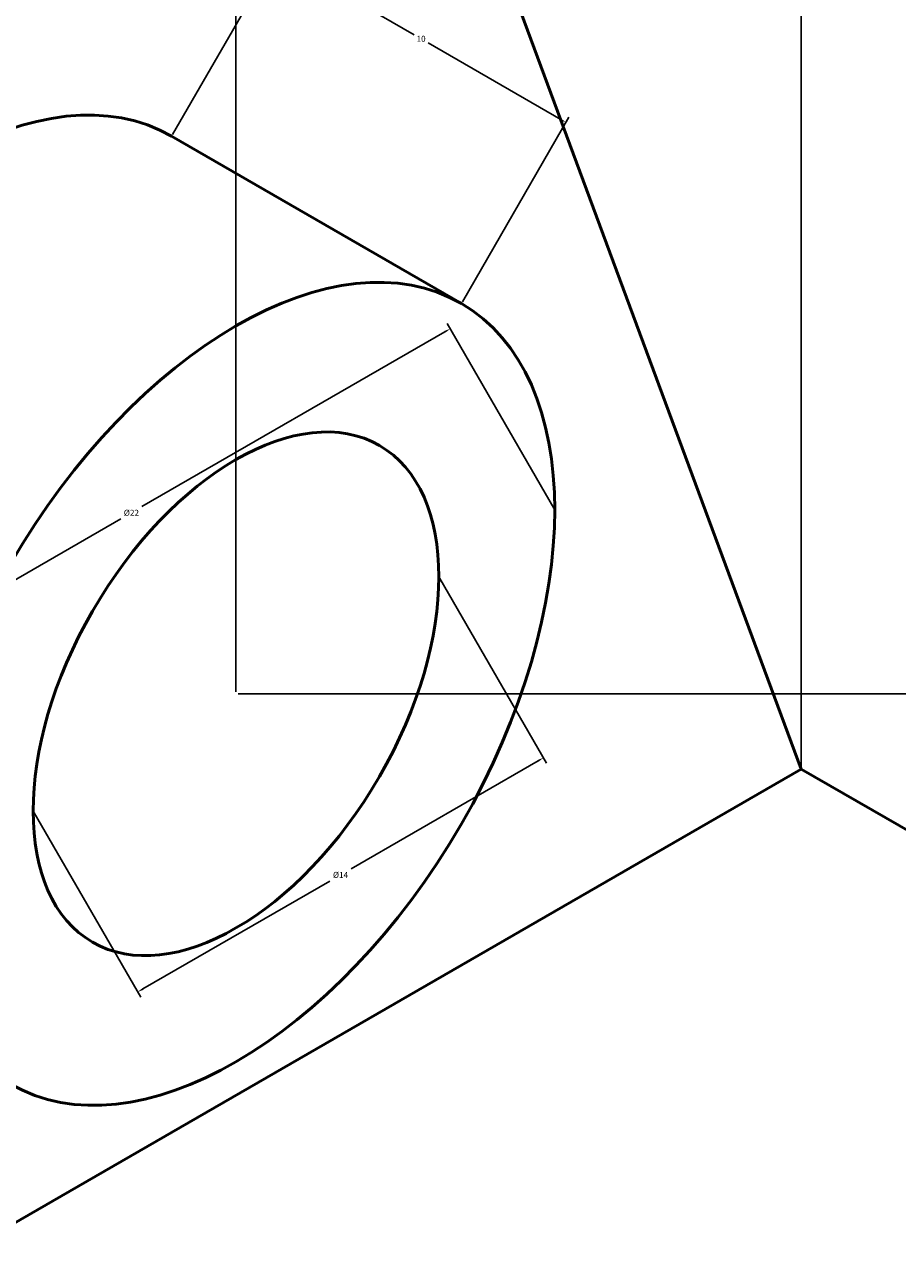
# Model space of a CAD drawing. Units: inches. Extents: x -23 to 69, y -27 to 96.
# Tile 7 of 10: x 11 to 37, y 35 to 72. Entities that reach past the tile are written whole.
import ezdxf

# ---------------------------------------------------------------- set-up
doc = ezdxf.new("R2010")
doc.units = ezdxf.units.IN
doc.header["$MEASUREMENT"] = 0
doc.layers.add('M-DIMS', color=2, linetype='Continuous', lineweight=18)
doc.layers.add('M-OUTL', color=7, linetype='Continuous', lineweight=50)
doc.styles.get("Standard").update_dxf_attribs({"font": 'arial.ttf'})
doc.dimstyles.get("Standard").update_dxf_attribs({"dimtxt": 0.18, "dimasz": 0.18, "dimexe": 0.18, "dimexo": 0.0625, "dimgap": 0.09, "dimtad": 0, "dimtih": 1, "dimtoh": 1, "dimdec": 4, "dimzin": 0, "dimdsep": 46, "dimtxsty": 'Standard', "dimcen": 0.09, "dimadec": 0, "dimazin": 0, "dimtfac": 1, "dimtdec": 4, "dimtofl": 0, "dimtmove": 0, "dimatfit": 3, "dimfxl": 1, "dimtolj": 1, "dimtzin": 0, "dimarcsym": 0})

# ---------------------------------------------------------------- blocks, each defined once
blk = doc.blocks.new('*D1')
at = {"layer": 'Defpoints', "color": 0, "transparency": 16777216}
for p in [(59.046, 39.281), (62.171, 33.869), (16.271, 7.369)]:
    blk.add_point(p, dxfattribs=at)
at = {"layer": 'M-DIMS', "color": 0, "lineweight": -2, "transparency": 16777216}
for p, q in [((62.139, 33.923), (58.956, 39.437)), ((58.89, 39.191), (36.315, 26.158)), ((13.302, 12.871), (35.877, 25.905)), ((16.24, 7.423), (13.056, 12.937))]:
    blk.add_line(p, q, dxfattribs=at)
at = {"layer": 'M-DIMS', "color": 0, "transparency": 16777216}
for points in [[(58.875, 39.217), (58.905, 39.165), (59.046, 39.281)], [(13.287, 12.897), (13.317, 12.845), (13.146, 12.781)]]:
    blk.add_solid(points, dxfattribs=at)
at = {"layer": 'M-DIMS', "color": 0, "transparency": 16777216, "insert": (36.096, 26.031), "char_height": 0.18, "attachment_point": 5}
blk.add_mtext('\\A1;53', dxfattribs=at)
blk = doc.blocks.new('*D10')
at = {"layer": 'Defpoints', "color": 0, "transparency": 16777216}
for p in [(27.431, 69.199), (15.646, 68.786), (24.306, 63.786)]:
    blk.add_point(p, dxfattribs=at)
at = {"layer": 'M-DIMS', "color": 0, "lineweight": -2, "transparency": 16777216}
for p, q in [((15.677, 68.84), (18.861, 74.354)), ((18.927, 74.109), (22.891, 71.82)), ((27.275, 69.289), (23.311, 71.577)), ((24.338, 63.84), (27.521, 69.354))]:
    blk.add_line(p, q, dxfattribs=at)
at = {"layer": 'M-DIMS', "color": 0, "transparency": 16777216}
for points in [[(18.942, 74.135), (18.912, 74.083), (18.771, 74.199)], [(27.29, 69.315), (27.26, 69.263), (27.431, 69.199)]]:
    blk.add_solid(points, dxfattribs=at)
at = {"layer": 'M-DIMS', "color": 0, "transparency": 16777216, "insert": (23.101, 71.699), "char_height": 0.18, "attachment_point": 5}
blk.add_mtext('\\A1;10', dxfattribs=at)
blk = doc.blocks.new('*D11')
at = {"layer": 'Defpoints', "color": 0, "transparency": 16777216}
for p in [(23.972, 63.031), (27.097, 57.619), (8.044, 46.619)]:
    blk.add_point(p, dxfattribs=at)
at = {"layer": 'M-DIMS', "color": 0, "lineweight": -2, "transparency": 16777216}
for p, q in [((23.816, 62.941), (14.761, 57.714)), ((27.065, 57.673), (23.882, 63.187)), ((5.075, 52.121), (14.129, 57.349)), ((8.013, 46.673), (4.829, 52.187))]:
    blk.add_line(p, q, dxfattribs=at)
at = {"layer": 'M-DIMS', "color": 0, "transparency": 16777216}
for points in [[(23.801, 62.967), (23.831, 62.915), (23.972, 63.031)], [(5.06, 52.147), (5.09, 52.095), (4.919, 52.031)]]:
    blk.add_solid(points, dxfattribs=at)
at = {"layer": 'M-DIMS', "color": 0, "transparency": 16777216, "insert": (14.445, 57.531), "char_height": 0.18, "attachment_point": 5}
blk.add_mtext('\\A1;%%c22', dxfattribs=at)
blk = doc.blocks.new('*D12')
at = {"layer": 'Defpoints', "color": 0, "transparency": 16777216}
for p in [(23.632, 55.619), (11.508, 48.619), (14.633, 43.206)]:
    blk.add_point(p, dxfattribs=at)
at = {"layer": 'M-DIMS', "color": 0, "lineweight": -2, "transparency": 16777216}
for p, q in [((23.664, 55.565), (26.847, 50.05)), ((26.602, 50.116), (21.012, 46.889)), ((11.539, 48.565), (14.723, 43.05)), ((14.789, 43.296), (20.379, 46.523))]:
    blk.add_line(p, q, dxfattribs=at)
at = {"layer": 'M-DIMS', "color": 0, "transparency": 16777216}
for points in [[(26.587, 50.142), (26.617, 50.09), (26.757, 50.206)], [(14.774, 43.322), (14.804, 43.27), (14.633, 43.206)]]:
    blk.add_solid(points, dxfattribs=at)
at = {"layer": 'M-DIMS', "color": 0, "transparency": 16777216, "insert": (20.695, 46.706), "char_height": 0.18, "attachment_point": 5}
blk.add_mtext('\\A1;%%c14', dxfattribs=at)
blk = doc.blocks.new('*D13')
at = {"layer": 'Defpoints', "color": 0, "transparency": 16777216}
for p in [(15.838, 89.119), (-22.888, -20.881), (36.623, -20.881)]:
    blk.add_point(p, dxfattribs=at)
at = {"layer": 'M-DIMS', "color": 0, "lineweight": -2, "transparency": 16777216}
for p, q in [((15.776, 89.119), (-23.068, 89.119)), ((-22.888, 88.939), (-22.888, 34.301)), ((-22.888, -20.701), (-22.888, 33.937)), ((36.56, -20.881), (-23.068, -20.881))]:
    blk.add_line(p, q, dxfattribs=at)
at = {"layer": 'M-DIMS', "color": 0, "transparency": 16777216}
for points in [[(-22.918, 88.939), (-22.858, 88.939), (-22.888, 89.119)], [(-22.918, -20.701), (-22.858, -20.701), (-22.888, -20.881)]]:
    blk.add_solid(points, dxfattribs=at)
at = {"layer": 'M-DIMS', "color": 0, "transparency": 16777216, "insert": (-22.888, 34.119), "char_height": 0.18, "attachment_point": 5}
blk.add_mtext('\\A1;110', dxfattribs=at)
blk = doc.blocks.new('*D14')
at = {"layer": 'Defpoints', "color": 0, "transparency": 16777216}
for p in [(21.034, 95.369), (21.034, 86.119), (34.458, 49.869)]:
    blk.add_point(p, dxfattribs=at)
at = {"layer": 'M-DIMS', "color": 0, "lineweight": -2, "transparency": 16777216}
for p, q in [((21.034, 86.181), (21.034, 95.549)), ((34.458, 49.931), (34.458, 95.549)), ((21.214, 95.369), (27.291, 95.369)), ((34.278, 95.369), (28.201, 95.369))]:
    blk.add_line(p, q, dxfattribs=at)
at = {"layer": 'M-DIMS', "color": 0, "transparency": 16777216}
for points in [[(21.214, 95.399), (21.214, 95.339), (21.034, 95.369)], [(34.278, 95.399), (34.278, 95.339), (34.458, 95.369)]]:
    blk.add_solid(points, dxfattribs=at)
at = {"layer": 'M-DIMS', "color": 0, "transparency": 16777216, "insert": (27.746, 95.369), "char_height": 0.18, "attachment_point": 5}
blk.add_mtext('\\A1;13.423', dxfattribs=at)
blk = doc.blocks.new('*D15')
at = {"layer": 'Defpoints', "color": 0, "transparency": 16777216}
for p in [(21.034, 86.119), (68.421, 86.119), (17.57, 52.119)]:
    blk.add_point(p, dxfattribs=at)
at = {"layer": 'M-DIMS', "color": 0, "lineweight": -2, "transparency": 16777216}
for p, q in [((21.097, 86.119), (68.601, 86.119)), ((68.421, 85.939), (68.421, 69.301)), ((68.421, 52.299), (68.421, 68.937)), ((17.633, 52.119), (68.601, 52.119))]:
    blk.add_line(p, q, dxfattribs=at)
at = {"layer": 'M-DIMS', "color": 0, "transparency": 16777216}
for points in [[(68.391, 85.939), (68.451, 85.939), (68.421, 86.119)], [(68.391, 52.299), (68.451, 52.299), (68.421, 52.119)]]:
    blk.add_solid(points, dxfattribs=at)
at = {"layer": 'M-DIMS', "color": 0, "transparency": 16777216, "insert": (68.421, 69.119), "char_height": 0.18, "attachment_point": 5}
blk.add_mtext('\\A1;34', dxfattribs=at)
blk = doc.blocks.new('*D16')
at = {"layer": 'Defpoints', "color": 0, "transparency": 16777216}
for p in [(17.57, 95.369), (-8.41, 69.119), (17.57, 52.119)]:
    blk.add_point(p, dxfattribs=at)
at = {"layer": 'M-DIMS', "color": 0, "lineweight": -2, "transparency": 16777216}
for p, q in [((-8.41, 69.181), (-8.41, 95.549)), ((17.57, 52.181), (17.57, 95.549)), ((-8.23, 95.369), (4.184, 95.369)), ((17.39, 95.369), (4.975, 95.369))]:
    blk.add_line(p, q, dxfattribs=at)
at = {"layer": 'M-DIMS', "color": 0, "transparency": 16777216}
for points in [[(-8.23, 95.399), (-8.23, 95.339), (-8.41, 95.369)], [(17.39, 95.399), (17.39, 95.339), (17.57, 95.369)]]:
    blk.add_solid(points, dxfattribs=at)
at = {"layer": 'M-DIMS', "color": 0, "transparency": 16777216, "insert": (4.58, 95.369), "char_height": 0.18, "attachment_point": 5}
blk.add_mtext('\\A1;25.98', dxfattribs=at)

msp = doc.modelspace()

# ---------------------------------------------------------------- linework, layer by layer
at = {"layer": 'M-OUTL'}
for p, q in [((21.0344, 86.1186), (34.4578, 49.8686)), ((15.6461, 68.7859), (24.3064, 63.7859)), ((34.4578, 49.8686), (-11.4416, 23.3686)), ((62.1706, 33.8686), (34.4578, 49.8686))]:
    msp.add_line(p, q, dxfattribs=at)
msp.add_ellipse((8.91, 57.1186), major_axis=(-6.7361, -11.6673), ratio=0.5773503, start_param=3.1415927, end_param=6.2831853, dxfattribs=at)
for major_axis in [(-6.7361, -11.6673), (-4.2866, -7.4246)]:
    msp.add_ellipse((17.5703, 52.1186), major_axis=major_axis, ratio=0.5773503, dxfattribs=at)

# ---------------------------------------------------------------- dimensions: what is measured, and where the dimension line sits
at = {"layer": 'M-DIMS'}
for base, p1, p2, override, picture, middle in [((17.5703, 95.3686), (-8.4105, 69.1186), (17.5703, 52.1186), {"dimdec": 2, "dimlfac": 1, "dimrnd": 0, "dimzin": 0, "dimdsep": 46, "dimlunit": 2}, '*D16', (4.5799, 95.3686)), ((21.0344, 95.3686), (34.4578, 49.8686), (21.0344, 86.1186), {"dimdec": 3, "dimlfac": 1, "dimrnd": 0, "dimzin": 0, "dimdsep": 46, "dimlunit": 2}, '*D14', (27.7461, 95.3686))]:
    dim = msp.add_linear_dim(base=base, p1=p1, p2=p2, dimstyle='Standard', override=override, dxfattribs=at)
    dim.commit()
    dim.dimension.update_dxf_attribs({"geometry": picture, "text_midpoint": middle})
for base, p1, p2, angle, picture, middle in [((-22.8877, -20.8814), (15.8382, 89.1186), (36.6228, -20.8814), 90, '*D13', (-22.8877, 34.1186)), ((68.4206, 86.1186), (17.5703, 52.1186), (21.0344, 86.1186), 90, '*D15', (68.4206, 69.1186)), ((27.4314, 69.1986), (15.6461, 68.7859), (24.3064, 63.7859), 330, '*D10', (23.1012, 71.6986)), ((59.0456, 39.2813), (16.2712, 7.3686), (62.1706, 33.8686), 30, '*D1', (36.0959, 26.0313))]:
    dim = msp.add_linear_dim(base=base, p1=p1, p2=p2, angle=angle, dimstyle='Standard', override={"dimdec": 0, "dimlfac": 1, "dimrnd": 0, "dimzin": 0, "dimdsep": 46, "dimlunit": 2}, dxfattribs=at)
    dim.commit()
    dim.dimension.update_dxf_attribs({"geometry": picture, "text_midpoint": middle})
for base, p1, p2, angle, picture, middle in [((23.9715, 63.0313), (8.044, 46.6186), (27.0965, 57.6186), 30, '*D11', (14.4453, 57.5313)), ((14.6331, 43.206), (23.6324, 55.6186), (11.5081, 48.6186), 210, '*D12', (20.6953, 46.706))]:
    dim = msp.add_linear_dim(base=base, p1=p1, p2=p2, angle=angle, text='%%c<>', dimstyle='Standard', override={"dimdec": 0, "dimlfac": 1, "dimrnd": 0, "dimzin": 0, "dimdsep": 46, "dimlunit": 2}, dxfattribs=at)
    dim.commit()
    dim.dimension.update_dxf_attribs({"geometry": picture, "text_midpoint": middle})

doc.saveas('drawing.dxf')
